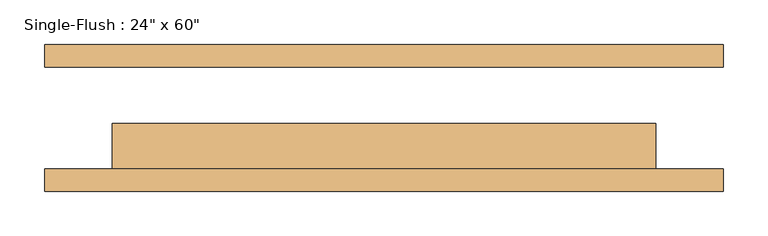
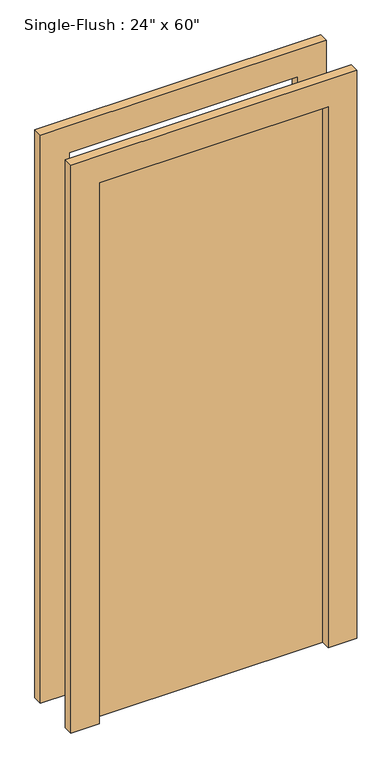
"""IFC4 building model written with IfcOpenShell, lengths in millimetres: door geometry."""

from ifc_helpers import new_model, si_unit, frame, origin, origin_with_axes, place, context, project, spatial, polyline, outline, extrude, source, transform, mapped, element, save


def door_bffbd567(model_context):
    return source(origin(), model_context, "Body", "SweptSolid", [
        extrude(outline(polyline([(1600.2, -381.0), (0.0, -381.0), (0.0, -304.8), (1524.0, -304.8), (1524.0, 304.8), (0.0, 304.8), (0.0, 381.0), (1600.2, 381.0), (1600.2, -381.0)])), frame((0.0, -82.55, 0.0), z_axis=(0.0, 1.0, 0.0), x_axis=(0.0, 0.0, 1.0)), (0.0, 0.0, 1.0), 25.4),
        extrude(outline(polyline([(1600.2, 381.0), (1600.2, -381.0), (0.0, -381.0), (0.0, -304.8), (1524.0, -304.8), (1524.0, 304.8), (0.0, 304.8), (0.0, 381.0), (1600.2, 381.0)])), frame((0.0, 57.15, 0.0), z_axis=(0.0, 1.0, 0.0), x_axis=(0.0, 0.0, 1.0)), (0.0, 0.0, 1.0), 25.4),
        extrude(outline(polyline([(304.8, -6.35), (304.8, -57.15), (-304.8, -57.15), (-304.8, -6.35), (304.8, -6.35)])), origin_with_axes(), (0.0, 0.0, 1.0), 1524.0),
    ])


if __name__ == "__main__":
    model = new_model("IFC4")
    model_context = context("Model", 3, world=origin())
    ifc_project = project(units=[si_unit("LENGTHUNIT", "METRE", prefix="MILLI")], contexts=[model_context])
    site = spatial("IfcSite", under=ifc_project)
    building = spatial("IfcBuilding", under=site)
    placement = place(None, origin())
    door_shape = door_bffbd567(model_context)
    element("IfcDoor", 1, ObjectType="Single-Flush : 24\" x 60\"", at=placement, inside=building, context=model_context, shape_type="MappedRepresentation", body=[
        mapped(door_shape, transform((0.0, 0.0, 0.0), x_axis=(1.0, 0.0, 0.0), y_axis=(0.0, 1.0, 0.0), z_axis=(0.0, 0.0, 1.0))),
    ])
    save(model, "model.ifc")

# Revit data of these elements
# Type "Single-Flush : 24\" x 60\""
#   Type Mark = "13"
#   Construction Type Id = "MDOOR"
#   Assembly Code = "C1020"
#   Analytic Construction = "Metal"
#   Thickness = 0' - 2"
#   Heat Transfer Coefficient (U) = 0.651978 BTU/(h·ft²·°F)
#   Height = 5' - 0"
#   Trim Projection Ext = 0' - 1"
#   Trim Projection Int = 0' - 1"
#   Trim Width = 0' - 3"
#   Width = 2' - 0"
#   Define Thermal Properties by = 1
#   Door Material = Door - Panel
#   Frame Material = Door - Frame
#   Visual Light Transmittance = 0
#   Solar Heat Gain Coefficient = 0
#   Function = (empty or 0)
#   Wall Closure = (empty or 0)
# Element 1 (IfcDoor, "Single-Flush : 24\" x 60\"")
#   Materials on its faces: "Door - Frame", "Door - Panel"
# Materials
#   "Door - Panel": class "Wood", colour RGB 210 159 95, transparency 0, Cost = 0
#   "Door - Frame": colour RGB 118 70 51, transparency 0, Cost = 0
